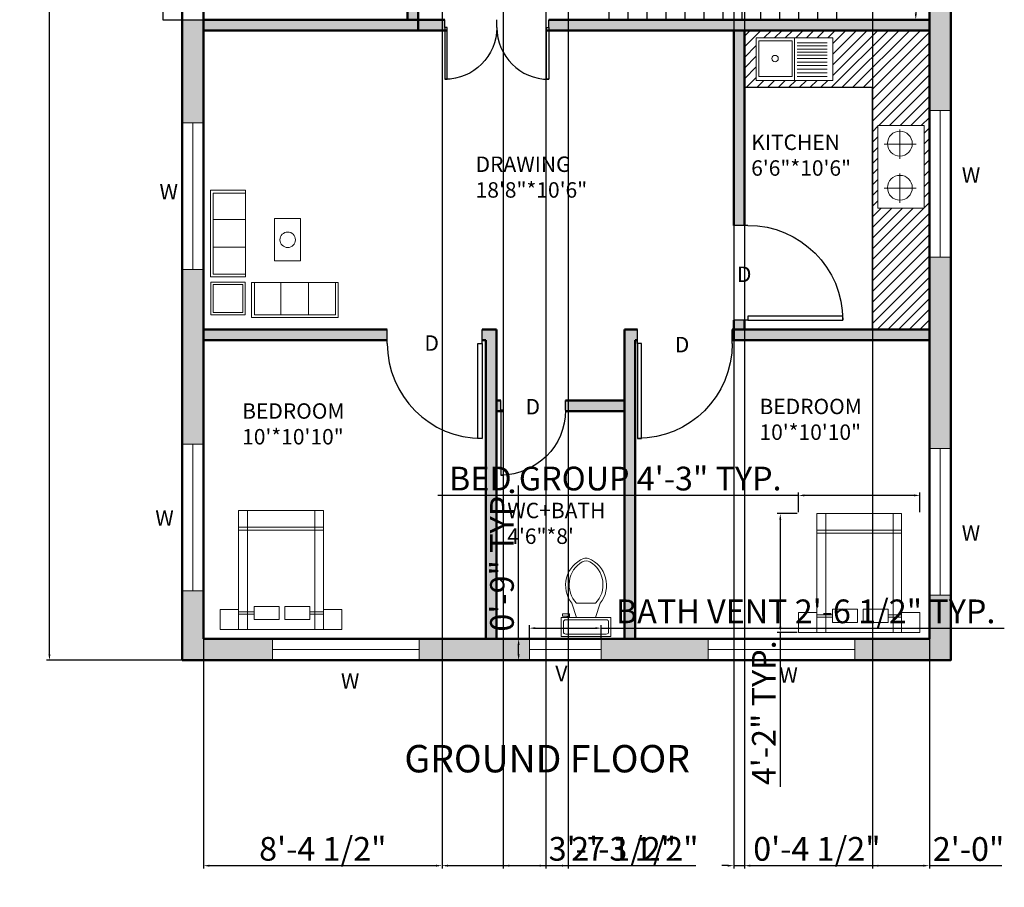
# Model space of a CAD drawing. Units: inches. Extents: x 1935 to 2445, y 1978 to 2806.
# Tile 1 of 4: x 1942 to 2357, y 1978 to 2344. Entities that reach past the tile are written whole.
import ezdxf

# ---------------------------------------------------------------- set-up
doc = ezdxf.new("R2010")
doc.units = ezdxf.units.IN
for name, color, linetype, lineweight in [('A-ANNO-DIMS', 2, 'Continuous', 18), ('A-ANNO-TEXT', 7, 'Continuous', 25), ('A-AREA-IDEN', 130, 'Continuous', 25), ('A-DOOR', 3, 'Continuous', 25), ('A-EQPM', 8, 'Continuous', 18), ('A-FLOR-CASE', 123, 'Continuous', 25), ('A-FLOR-CASE-PATT', 123, 'Continuous', 13), ('A-FLOR-FIXT', 9, 'Continuous', 18), ('A-FLOR-OTLN', 7, 'Continuous', 25), ('A-FLOR-STRS', 7, 'Continuous', 25), ('A-FURN', 9, 'Continuous', 18), ('A-GLAZ', 4, 'Continuous', 18), ('A-WALL-PATT', 225, 'Continuous', 13), ('SOFA', 10, 'Continuous', 18), ('WALL', 225, 'Continuous', 50)]:
    doc.layers.add(name, color=color, linetype=linetype, lineweight=lineweight)
doc.styles.get("Standard").update_dxf_attribs({"font": 'arial.ttf'})
doc.dimstyles.new('ISO-25', dxfattribs={"dimtxt": 10, "dimasz": 2.5, "dimexe": 1.25, "dimexo": 0.625, "dimtad": 1, "dimdec": 0, "dimlunit": 4, "dimtxsty": 'Standard', "dimcen": 2.5, "dimadec": 0, "dimazin": 0, "dimtfac": 1, "dimtdec": 0, "dimtmove": 0, "dimatfit": 3, "dimfxl": 1, "dimarcsym": 0})

# ---------------------------------------------------------------- blocks, each defined once
blk = doc.blocks.new('*U2')
for p, q in [((0, 0), (0, -6)), ((40, 0), (40, -6))]:
    blk.add_line(p, q)
blk.add_lwpolyline([(0, 0), (0, 40), (1.75, 40), (1.75, 0)], close=True)
blk.add_arc((0, 0), 40, 0, 90)
blk = doc.blocks.new('*U4')
for p, q in [((9.5, -6), (9.5, -2)), ((-8, -8.5), (-8, -8)), ((-7, -8), (-7, -9.5)), ((-4, -8), (-6, -14)), ((4, -8), (6, -14)), ((-10, -8.5), (-8, -8.5)), ((-10, -9.5), (-10, -8.5)), ((-7, -9.5), (-10, -9.5)), ((4, -14), (-4, -14))]:
    blk.add_line(p, q)
blk.add_lwpolyline([(10.5, -8), (10.5, 0), (-10.5, 0), (-10.5, -8)], close=True)
for points in [[(-9.5, -2), (-9.5, -6)], [(8.5, -1), (-8.5, -1)], [(-8.5, -7), (8.5, -7)]]:
    blk.add_lwpolyline(points)
for centre, radius, start, end in [((-8.62, -1.88), 0.884, 81.8699, 188.1301), ((8.62, -1.88), 0.884, 351.8699, 98.1301), ((-8.62, -6.12), 0.884, 171.8699, 278.1301), ((8.62, -6.12), 0.884, 261.8699, 8.1301), ((3.52, -21.58), 12.17, 141.4691, 247.9714), ((4.2, -21.82), 11.33, 136.3677, 238.9468), ((-3.52, -21.58), 12.17, 292.0284, 38.5307), ((-4.2, -21.82), 11.33, 301.053, 43.6321), ((0, -27.88), 4, 245.7318, 294.2682), ((0, -29), 4, 254.8605, 285.1395)]:
    blk.add_arc(centre, radius, start, end)
blk = doc.blocks.new('*D7')
at = {"layer": 'A-ANNO-DIMS', "color": 0, "lineweight": -2, "transparency": 16777216}
for p, q in [((2324.56, 2423.88), (2318.18, 2423.88)), ((2319.43, 2421.38), (2319.43, 2346.38)), ((2324.56, 2343.88), (2318.18, 2343.88))]:
    blk.add_line(p, q, dxfattribs=at)
at = {"layer": 'A-ANNO-DIMS', "color": 0, "lineweight": 100, "transparency": 16777216}
for points in [[(2319.01, 2421.38), (2319.85, 2421.38), (2319.43, 2423.88)], [(2319.01, 2346.38), (2319.85, 2346.38), (2319.43, 2343.88)]]:
    blk.add_solid(points, dxfattribs=at)
at = {"layer": 'Defpoints', "color": 0, "lineweight": 100, "transparency": 16777216}
for p in [(2325.18, 2423.88), (2319.43, 2343.88), (2325.18, 2343.88)]:
    blk.add_point(p, dxfattribs=at)
at = {"layer": 'A-ANNO-DIMS', "color": 0, "transparency": 16777216, "insert": (2313.7, 2383.88), "char_height": 10, "attachment_point": 5, "rotation": 90}
blk.add_mtext('6\'-8"', dxfattribs=at)
blk = doc.blocks.new('*D9')
at = {"layer": 'A-ANNO-DIMS', "color": 0, "lineweight": -2, "transparency": 16777216}
for p, q in [((2333.56, 2697.88), (1952.98, 2697.88)), ((1954.23, 2076.38), (1954.23, 2695.38)), ((2333.56, 2073.88), (1952.98, 2073.88))]:
    blk.add_line(p, q, dxfattribs=at)
at = {"layer": 'A-ANNO-DIMS', "color": 0, "lineweight": 100, "transparency": 16777216}
for points in [[(1953.82, 2695.38), (1954.65, 2695.38), (1954.23, 2697.88)], [(1953.82, 2076.38), (1954.65, 2076.38), (1954.23, 2073.88)]]:
    blk.add_solid(points, dxfattribs=at)
at = {"layer": 'Defpoints', "color": 0, "lineweight": 100, "transparency": 16777216}
for p in [(1954.23, 2697.88), (2334.18, 2697.88), (2334.18, 2073.88)]:
    blk.add_point(p, dxfattribs=at)
at = {"layer": 'A-ANNO-DIMS', "color": 0, "transparency": 16777216, "insert": (1948.5, 2385.88), "char_height": 10, "attachment_point": 5, "rotation": 90}
blk.add_mtext("52'", dxfattribs=at)
blk = doc.blocks.new('WINDOW-STD')
blk.add_line((0, 4.5), (61.82, 4.5))
blk.add_lwpolyline([(0, 9), (61.82, 9), (61.82, 0), (0, 0)], close=True)
blk = doc.blocks.new('VENT-BATH')
blk.add_line((0, 4.5), (30.29, 4.5))
blk.add_lwpolyline([(0, 0), (30.29, 0), (30.29, 9), (0, 9)], close=True)
blk = doc.blocks.new('BED-WITH-NIGHTSTANDS')
for p, q in [((11.32, 50.11), (11.32, 0)), ((39.64, 0), (39.64, 50.11)), ((13.46, 43.65), (7.73, 43.65)), ((13.46, 42.6), (7.73, 42.6)), ((43.47, 43.65), (36.85, 43.65)), ((43.47, 42.6), (36.85, 42.6)), ((7.73, 8.18), (43.47, 8.18)), ((7.73, 6.93), (43.47, 6.93)), ((43.47, 0), (39.64, 0))]:
    blk.add_line(p, q)
for points in [[(0, 50.11), (7.73, 50.11), (7.73, 41.64), (0, 41.64)], [(7.73, 50.11), (43.47, 50.11), (43.47, 0), (7.73, 0)], [(43.47, 50.11), (51.2, 50.11), (51.2, 41.64), (43.47, 41.64)], [(13.46, 45.91), (23.93, 45.91), (23.93, 40.33), (13.46, 40.33)], [(26.4, 45.91), (36.86, 45.91), (36.86, 40.33), (26.4, 40.33)]]:
    blk.add_lwpolyline(points, close=True)
blk = doc.blocks.new('SOFA-3-SEAT')
for p, q in [((0, 0), (0, 14.72)), ((0, 14.72), (36.65, 14.72)), ((12.37, 13.53), (12.37, 0)), ((24.09, 13.53), (24.09, 0)), ((36.65, 14.72), (36.65, 0)), ((1.26, 0), (0, 0)), ((36.65, 0), (31.67, 0))]:
    blk.add_line(p, q)
blk.add_lwpolyline([(1.26, 0), (35.43, 0), (35.43, 13.53), (1.26, 13.53)], close=True)
blk = doc.blocks.new('TABLE-END')
for points in [[(0, 13.76), (14.51, 13.76), (14.51, 0), (0, 0)], [(1, 12.76), (13.51, 12.76), (13.51, 1), (1, 1)]]:
    blk.add_lwpolyline(points, close=True)
blk = doc.blocks.new('TABLE-COFFEE')
blk.add_lwpolyline([(0, 0), (10.92, 0), (10.92, 17.81), (0, 17.81)], close=True)
blk.add_circle((5.5, 9), 3.27)
blk = doc.blocks.new('SINK-WITH-DRAINBOARD')
for p, q in [((16.15, 17.9), (16.15, 0)), ((17.28, 15.79), (29.84, 15.79)), ((17.28, 14.55), (29.84, 14.55)), ((17.28, 13.18), (29.84, 13.18)), ((17.28, 11.91), (29.84, 11.91)), ((17.28, 10.66), (29.84, 10.66)), ((17.28, 9.26), (29.84, 9.26)), ((17.28, 7.74), (29.84, 7.74)), ((17.28, 6.29), (29.84, 6.29)), ((17.28, 4.78), (29.84, 4.78)), ((17.28, 3.21), (29.84, 3.21)), ((17.28, 1.68), (29.84, 1.68))]:
    blk.add_line(p, q)
for points in [[(0, 17.9), (32.3, 17.9), (32.3, 0), (0, 0)], [(1.08, 1.69), (15.15, 1.69), (15.15, 16.69), (1.08, 16.69)]]:
    blk.add_lwpolyline(points, close=True)
blk.add_circle((7.93, 9.19), 1.34)
blk = doc.blocks.new('COOKTOP-2-BURNER')
for p, q in [((9.23, 27.22), (9.23, 33.16)), ((9.23, 33.16), (9.23, 20.87)), ((9.23, 27.02), (2.64, 27.02)), ((2.64, 27.02), (16.07, 27.02)), ((9.23, 20.87), (9.23, 27.02)), ((9.23, 8.61), (9.23, 14.56)), ((9.23, 14.56), (9.23, 2.26)), ((9.23, 8.41), (2.64, 8.41)), ((2.64, 8.41), (16.07, 8.41)), ((9.23, 2.26), (9.23, 8.41))]:
    blk.add_line(p, q)
blk.add_lwpolyline([(0, 34.88), (19.51, 34.88), (19.51, 0), (0, 0)], close=True)
for centre in [(9.23, 27.22), (9.23, 8.61)]:
    blk.add_circle(centre, 5.23)
blk = doc.blocks.new('*D20')
at = {"layer": 'A-ANNO-DIMS', "color": 0, "lineweight": -2, "transparency": 16777216}
for p, q in [((2270, 2143.39), (2118.02, 2143.39)), ((2270, 2136.33), (2270, 2144.64)), ((2318.7, 2143.39), (2272.5, 2143.39)), ((2321.2, 2136.33), (2321.2, 2144.64))]:
    blk.add_line(p, q, dxfattribs=at)
at = {"layer": 'A-ANNO-DIMS', "color": 0, "lineweight": 100, "transparency": 16777216}
for points in [[(2272.5, 2143.81), (2272.5, 2142.97), (2270, 2143.39)], [(2318.7, 2143.81), (2318.7, 2142.97), (2321.2, 2143.39)]]:
    blk.add_solid(points, dxfattribs=at)
at = {"layer": 'Defpoints', "color": 0, "lineweight": 100, "transparency": 16777216}
for p in [(2270, 2143.39), (2270, 2135.71), (2321.2, 2135.71)]:
    blk.add_point(p, dxfattribs=at)
at = {"layer": 'A-ANNO-DIMS', "color": 0, "transparency": 16777216, "insert": (2192.76, 2149.19), "char_height": 10, "attachment_point": 5}
blk.add_mtext('BED GROUP 4\'-3" TYP.', dxfattribs=at)
blk = doc.blocks.new('*D21')
at = {"layer": 'A-ANNO-DIMS', "color": 0, "lineweight": -2, "transparency": 16777216}
for p, q in [((2269.37, 2135.71), (2261.07, 2135.71)), ((2262.32, 2133.21), (2262.32, 2088.1)), ((2269.37, 2085.6), (2261.07, 2085.6)), ((2262.32, 2085.6), (2262.32, 2020.49))]:
    blk.add_line(p, q, dxfattribs=at)
at = {"layer": 'A-ANNO-DIMS', "color": 0, "lineweight": 100, "transparency": 16777216}
for points in [[(2261.9, 2133.21), (2262.73, 2133.21), (2262.32, 2135.71)], [(2261.9, 2088.1), (2262.73, 2088.1), (2262.32, 2085.6)]]:
    blk.add_solid(points, dxfattribs=at)
at = {"layer": 'Defpoints', "color": 0, "lineweight": 100, "transparency": 16777216}
for p in [(2270, 2135.71), (2262.32, 2085.6), (2270, 2085.6)]:
    blk.add_point(p, dxfattribs=at)
at = {"layer": 'A-ANNO-DIMS', "color": 0, "transparency": 16777216, "insert": (2256.67, 2051.79), "char_height": 10, "attachment_point": 5, "rotation": 90}
blk.add_mtext('4\'-2" TYP.', dxfattribs=at)
blk = doc.blocks.new('*D22')
at = {"layer": 'A-ANNO-DIMS', "color": 0, "lineweight": -2, "transparency": 16777216}
for p, q in [((2156.55, 2083.51), (2156.55, 2088.68)), ((2186.84, 2083.51), (2186.84, 2088.68)), ((2159.05, 2087.43), (2184.34, 2087.43)), ((2186.84, 2087.43), (2356.68, 2087.43))]:
    blk.add_line(p, q, dxfattribs=at)
at = {"layer": 'A-ANNO-DIMS', "color": 0, "lineweight": 100, "transparency": 16777216}
for points in [[(2159.05, 2087.84), (2159.05, 2087.01), (2156.55, 2087.43)], [(2184.34, 2087.84), (2184.34, 2087.01), (2186.84, 2087.43)]]:
    blk.add_solid(points, dxfattribs=at)
at = {"layer": 'Defpoints', "color": 0, "lineweight": 100, "transparency": 16777216}
for p in [(2186.84, 2087.43), (2156.55, 2082.88), (2186.84, 2082.88)]:
    blk.add_point(p, dxfattribs=at)
at = {"layer": 'A-ANNO-DIMS', "color": 0, "transparency": 16777216, "insert": (2273.01, 2093.22), "char_height": 10, "attachment_point": 5}
blk.add_mtext('BATH VENT 2\'-6 1/2" TYP.', dxfattribs=at)
blk = doc.blocks.new('*D23')
at = {"layer": 'A-ANNO-DIMS', "color": 0, "lineweight": -2, "transparency": 16777216}
for p, q in [((2152.01, 2082.88), (2152.01, 2147.59)), ((2155.93, 2082.88), (2150.76, 2082.88)), ((2152.01, 2076.38), (2152.01, 2080.38)), ((2155.93, 2073.88), (2150.76, 2073.88))]:
    blk.add_line(p, q, dxfattribs=at)
at = {"layer": 'A-ANNO-DIMS', "color": 0, "lineweight": 100, "transparency": 16777216}
for points in [[(2151.59, 2080.38), (2152.42, 2080.38), (2152.01, 2082.88)], [(2151.59, 2076.38), (2152.42, 2076.38), (2152.01, 2073.88)]]:
    blk.add_solid(points, dxfattribs=at)
at = {"layer": 'Defpoints', "color": 0, "lineweight": 100, "transparency": 16777216}
for p in [(2152.01, 2082.88), (2156.55, 2082.88), (2156.55, 2073.88)]:
    blk.add_point(p, dxfattribs=at)
at = {"layer": 'A-ANNO-DIMS', "color": 0, "transparency": 16777216, "insert": (2146.28, 2116.49), "char_height": 10, "attachment_point": 5, "rotation": 90}
blk.add_mtext('0\'-9" TYP.', dxfattribs=at)
blk = doc.blocks.new('*D39')
at = {"layer": 'A-ANNO-DIMS', "color": 0, "lineweight": -2, "transparency": 16777216}
for p, q in [((2019.18, 2423.26), (2019.18, 1986.08)), ((2119.73, 2423.26), (2119.73, 1986.08)), ((2021.68, 1987.33), (2117.23, 1987.33))]:
    blk.add_line(p, q, dxfattribs=at)
at = {"layer": 'A-ANNO-DIMS', "color": 0, "lineweight": 100, "transparency": 16777216}
for points in [[(2021.68, 1987.74), (2021.68, 1986.91), (2019.18, 1987.33)], [(2117.23, 1987.74), (2117.23, 1986.91), (2119.73, 1987.33)]]:
    blk.add_solid(points, dxfattribs=at)
at = {"layer": 'Defpoints', "color": 0, "lineweight": 100, "transparency": 16777216}
for p in [(2019.18, 2423.88), (2119.73, 2423.88), (2119.73, 1987.33)]:
    blk.add_point(p, dxfattribs=at)
at = {"layer": 'A-ANNO-DIMS', "color": 0, "transparency": 16777216, "insert": (2069.46, 1993.12), "char_height": 10, "attachment_point": 5}
blk.add_mtext('8\'-4 1/2"', dxfattribs=at)
blk = doc.blocks.new('*D40')
at = {"layer": 'A-ANNO-DIMS', "color": 0, "lineweight": -2, "transparency": 16777216}
for p, q in [((2119.73, 2423.26), (2119.73, 1986.08)), ((2163.45, 2423.26), (2163.45, 1986.08)), ((2122.23, 1987.33), (2160.95, 1987.33)), ((2163.45, 1987.33), (2217.08, 1987.33))]:
    blk.add_line(p, q, dxfattribs=at)
at = {"layer": 'A-ANNO-DIMS', "color": 0, "lineweight": 100, "transparency": 16777216}
for points in [[(2122.23, 1987.74), (2122.23, 1986.91), (2119.73, 1987.33)], [(2160.95, 1987.74), (2160.95, 1986.91), (2163.45, 1987.33)]]:
    blk.add_solid(points, dxfattribs=at)
at = {"layer": 'Defpoints', "color": 0, "lineweight": 100, "transparency": 16777216}
for p in [(2119.73, 2423.88), (2163.45, 2423.88), (2163.45, 1987.33)]:
    blk.add_point(p, dxfattribs=at)
at = {"layer": 'A-ANNO-DIMS', "color": 0, "transparency": 16777216, "insert": (2191.52, 1993.13), "char_height": 10, "attachment_point": 5}
blk.add_mtext('3\'-7 1/2"', dxfattribs=at)
blk = doc.blocks.new('*D42')
at = {"layer": 'A-ANNO-DIMS', "color": 0, "lineweight": -2, "transparency": 16777216}
for p, q in [((2145.55, 2591.86), (2145.55, 1986.08)), ((2172.86, 2592.26), (2172.86, 1986.08)), ((2148.05, 1987.33), (2170.36, 1987.33)), ((2172.86, 1987.33), (2226.66, 1987.33))]:
    blk.add_line(p, q, dxfattribs=at)
at = {"layer": 'A-ANNO-DIMS', "color": 0, "lineweight": 100, "transparency": 16777216}
for points in [[(2148.05, 1987.74), (2148.05, 1986.91), (2145.55, 1987.33)], [(2170.36, 1987.74), (2170.36, 1986.91), (2172.86, 1987.33)]]:
    blk.add_solid(points, dxfattribs=at)
at = {"layer": 'Defpoints', "color": 0, "lineweight": 100, "transparency": 16777216}
for p in [(2145.55, 2592.49), (2172.86, 2592.88), (2172.86, 1987.33)]:
    blk.add_point(p, dxfattribs=at)
at = {"layer": 'A-ANNO-DIMS', "color": 0, "transparency": 16777216, "insert": (2201.01, 1993.13), "char_height": 10, "attachment_point": 5}
blk.add_mtext('2\'-3 1/2"', dxfattribs=at)
blk = doc.blocks.new('*D44')
at = {"layer": 'A-ANNO-DIMS', "color": 0, "lineweight": -2, "transparency": 16777216}
for p, q in [((2325.18, 2454.54), (2325.18, 1986.08)), ((2301.18, 2451.76), (2301.18, 1986.08)), ((2303.68, 1987.33), (2322.68, 1987.33)), ((2325.18, 1987.33), (2355.69, 1987.33))]:
    blk.add_line(p, q, dxfattribs=at)
at = {"layer": 'A-ANNO-DIMS', "color": 0, "lineweight": 100, "transparency": 16777216}
for points in [[(2303.68, 1987.74), (2303.68, 1986.91), (2301.18, 1987.33)], [(2322.68, 1987.74), (2322.68, 1986.91), (2325.18, 1987.33)]]:
    blk.add_solid(points, dxfattribs=at)
at = {"layer": 'Defpoints', "color": 0, "lineweight": 100, "transparency": 16777216}
for p in [(2325.18, 2455.16), (2301.18, 2452.38), (2325.18, 1987.33)]:
    blk.add_point(p, dxfattribs=at)
at = {"layer": 'A-ANNO-DIMS', "color": 0, "transparency": 16777216, "insert": (2341.69, 1993.06), "char_height": 10, "attachment_point": 5}
blk.add_mtext('2\'-0"', dxfattribs=at)
blk = doc.blocks.new('*D45')
at = {"layer": 'A-ANNO-DIMS', "color": 0, "lineweight": -2, "transparency": 16777216}
for p, q in [((2242.68, 2510.08), (2242.68, 1986.08)), ((2247.18, 2510.08), (2247.18, 1986.08)), ((2240.18, 1987.33), (2237.68, 1987.33)), ((2242.68, 1987.33), (2247.18, 1987.33)), ((2249.68, 1987.33), (2303.32, 1987.33))]:
    blk.add_line(p, q, dxfattribs=at)
at = {"layer": 'A-ANNO-DIMS', "color": 0, "lineweight": 100, "transparency": 16777216}
for points in [[(2240.18, 1987.74), (2240.18, 1986.91), (2242.68, 1987.33)], [(2249.68, 1987.74), (2249.68, 1986.91), (2247.18, 1987.33)]]:
    blk.add_solid(points, dxfattribs=at)
at = {"layer": 'Defpoints', "color": 0, "lineweight": 100, "transparency": 16777216}
for p in [(2242.68, 2510.71), (2247.18, 2510.71), (2247.18, 1987.33)]:
    blk.add_point(p, dxfattribs=at)
at = {"layer": 'A-ANNO-DIMS', "color": 0, "transparency": 16777216, "insert": (2277.75, 1993.12), "char_height": 10, "attachment_point": 5}
blk.add_mtext('0\'-4 1/2"', dxfattribs=at)

msp = doc.modelspace()

# ---------------------------------------------------------------- hatches: boundary and pattern name
at = {"layer": 'A-FLOR-CASE-PATT'}
h = msp.add_hatch(dxfattribs=at)
h.set_pattern_fill('ANSI31', color=256)
h.paths.add_polyline_path([(2325.18, 2339.38), (2286.18, 2339.38), (2247.18, 2339.38), (2247.18, 2315.38), (2301.18, 2315.38), (2301.18, 2213.38), (2325.18, 2213.38)])
h.paths.add_polyline_path([(2284.48, 2318.31), (2252.19, 2318.31), (2252.19, 2336.21), (2284.48, 2336.21)], flags=16)
h.paths.add_polyline_path([(2303.5, 2299.32), (2323.01, 2299.32), (2323.01, 2264.44), (2303.5, 2264.44)], flags=16)
h.paths.add_polyline_path([(2317.96, 2291.66, -1), (2307.51, 2291.66, -1)], flags=0)
h.paths.add_polyline_path([(2267.33, 2320), (2253.26, 2320), (2253.26, 2335.01), (2267.33, 2335.01)], flags=0)
h.paths.add_polyline_path([(2258.78, 2327.5, -1), (2261.46, 2327.5, -1)], flags=0)
h.paths.add_polyline_path([(2317.96, 2273.05, -1), (2307.51, 2273.05, -1)], flags=0)
h.paths.add_polyline_path([(2325.18, 2554.38), (2301.18, 2554.38), (2301.18, 2452.38), (2247.18, 2452.38), (2247.18, 2428.38), (2325.18, 2428.38)])
h.paths.add_polyline_path([(2323.01, 2511.98), (2323.01, 2477.1), (2303.5, 2477.1), (2303.5, 2511.98)], flags=16)
h.paths.add_polyline_path([(2317.96, 2504.31, -1), (2307.51, 2504.31, -1)], flags=0)
h.paths.add_polyline_path([(2317.96, 2485.7, -1), (2307.51, 2485.7, -1)], flags=0)
h.paths.add_polyline_path([(2284.48, 2450.03), (2284.48, 2432.13), (2252.19, 2432.13), (2252.19, 2450.03)], flags=16)
h.paths.add_polyline_path([(2267.33, 2448.82), (2267.33, 2433.82), (2253.26, 2433.82), (2253.26, 2448.82)], flags=0)
h.paths.add_polyline_path([(2261.46, 2441.32, -1), (2258.78, 2441.32, -1)], flags=0)
at = {"layer": 'A-WALL-PATT'}
h = msp.add_hatch(color=256, dxfattribs=at)
h.dxf.hatch_style = 1
h.paths.add_polyline_path([(2047.95, 2697.88), (2010.18, 2697.88), (2010.18, 2654.96), (2019.18, 2654.96), (2019.18, 2688.88), (2047.95, 2688.88)], flags=16)
h.paths.add_polyline_path([(2156.17, 2697.88), (2109.77, 2697.88), (2109.77, 2688.88), (2139.18, 2688.88), (2156.17, 2688.88)], flags=17)
h.paths.add_polyline_path([(2231.53, 2697.88), (2186.46, 2697.88), (2186.46, 2688.88), (2231.53, 2688.88)], flags=17)
h.paths.add_polyline_path([(2334.18, 2697.88), (2293.35, 2697.88), (2293.35, 2688.88), (2325.18, 2688.88), (2325.18, 2651.52), (2334.18, 2651.52)], flags=17)
h.paths.add_polyline_path([(2247.18, 2554.38), (2242.68, 2554.38), (2242.68, 2550.71), (2247.18, 2550.71)], flags=17)
h.paths.add_polyline_path([(2145.55, 2592.49), (2145.55, 2592.88), (2143.68, 2592.88), (2143.68, 2588.39), (2145.55, 2588.39)], flags=17)
h.paths.add_polyline_path([(2197.68, 2592.88), (2172.86, 2592.88, -0.003651), (2172.86, 2592.49), (2172.86, 2588.39), (2197.68, 2588.39)], flags=17)
h.paths.add_polyline_path([(2203.16, 2558.88), (2137.4, 2558.88), (2137.4, 2554.38), (2143.68, 2554.38), (2203.16, 2554.38)], flags=17)
h.paths.add_polyline_path([(2097.4, 2558.88), (2019.18, 2558.88), (2019.18, 2554.38), (2097.4, 2554.38)], flags=17)
h.paths.add_polyline_path([(2143.68, 2688.88), (2139.18, 2688.88), (2139.18, 2558.88), (2143.68, 2558.88)], flags=17)
h.paths.add_polyline_path([(2202.18, 2688.88), (2197.68, 2688.88), (2197.68, 2592.88), (2197.68, 2588.39), (2197.68, 2558.88), (2202.18, 2558.88), (2202.18, 2588.38)], flags=17)
h.paths.add_polyline_path([(2241.74, 2229.79), (2251.55, 2229.79), (2251.55, 2243.19), (2241.74, 2243.19)], flags=25)
h.paths.add_polyline_path([(2215.53, 2200.14), (2225.34, 2200.14), (2225.34, 2213.54), (2215.53, 2213.54)], flags=25)
h.paths.add_polyline_path([(2152.61, 2173.98), (2162.42, 2173.98), (2162.42, 2187.38), (2152.61, 2187.38)], flags=25)
h.paths.add_polyline_path([(2109.99, 2200.78), (2119.8, 2200.78), (2119.8, 2214.18), (2109.99, 2214.18)], flags=25)
h.paths.add_polyline_path([(2139.65, 2343.23), (2149.46, 2343.23), (2149.46, 2356.63), (2139.65, 2356.63)], flags=25)
h.paths.add_polyline_path([(2138.05, 2412.22), (2147.87, 2412.22), (2147.87, 2425.62), (2138.05, 2425.62)], flags=25)
h.paths.add_polyline_path([(2242.1, 2526.57), (2251.91, 2526.57), (2251.91, 2539.97), (2242.1, 2539.97)], flags=25)
h.paths.add_polyline_path([(2212.92, 2555.35), (2222.74, 2555.35), (2222.74, 2568.75), (2212.92, 2568.75)], flags=25)
h.paths.add_polyline_path([(2111.94, 2553.1), (2121.75, 2553.1), (2121.75, 2566.5), (2111.94, 2566.5)], flags=25)
h.paths.add_polyline_path([(2032.85, 2161.17), (2083.36, 2161.17), (2083.36, 2185.43), (2032.85, 2185.43)], flags=25)
h.paths.add_polyline_path([(2145.49, 2119.25), (2193.41, 2119.25), (2193.41, 2143.52), (2145.49, 2143.52)], flags=25)
h.paths.add_polyline_path([(2250.93, 2163.1), (2301.44, 2163.1), (2301.44, 2187.36), (2250.93, 2187.36)], flags=25)
h.paths.add_polyline_path([(2247.75, 2274.43), (2290.88, 2274.43), (2290.88, 2298.69), (2247.75, 2298.69)], flags=25)
h.paths.add_polyline_path([(2131.26, 2265.2), (2178.71, 2265.2), (2178.71, 2289.46), (2131.26, 2289.46)], flags=25)
h.paths.add_polyline_path([(2092.71, 2400.61), (2092.71, 2376.16), (2106.11, 2376.16), (2106.11, 2400.61)], flags=25)
h.paths.add_polyline_path([(2173.61, 2396.23), (2189.48, 2396.23), (2189.48, 2409.63), (2173.61, 2409.63)], flags=25)
h.paths.add_polyline_path([(2028.85, 2376.01), (2076.42, 2376.01), (2076.42, 2400.28), (2028.85, 2400.28)], flags=25)
h.paths.add_polyline_path([(2135.3, 2481.1), (2182.75, 2481.1), (2182.75, 2505.37), (2135.3, 2505.37)], flags=25)
h.paths.add_polyline_path([(2249.01, 2476.21), (2292.13, 2476.21), (2292.13, 2500.47), (2249.01, 2500.47)], flags=25)
h.paths.add_polyline_path([(2251.9, 2596.84), (2302.42, 2596.84), (2302.42, 2621.11), (2251.9, 2621.11)], flags=25)
h.paths.add_polyline_path([(2030.66, 2589.83), (2081.18, 2589.83), (2081.18, 2614.09), (2030.66, 2614.09)], flags=25)
h.paths.add_polyline_path([(2019.18, 2593.14), (2010.18, 2593.14), (2010.18, 2520.31), (2019.18, 2520.31)])
h.paths.add_polyline_path([(2010.18, 2164.99), (2019.18, 2164.99), (2019.18, 2238.56), (2010.18, 2238.56)])
h.paths.add_polyline_path([(2048.33, 2073.88), (2048.33, 2082.88), (2019.18, 2082.88), (2019.18, 2103.18), (2010.18, 2103.18), (2010.18, 2073.88)])
h.paths.add_polyline_path([(2156.55, 2073.88), (2156.55, 2082.88), (2110.15, 2082.88), (2110.15, 2073.88)])
h.paths.add_polyline_path([(2231.91, 2073.88), (2231.91, 2082.88), (2186.84, 2082.88), (2186.84, 2073.88)])
h.paths.add_polyline_path([(2047.95, 2688.88), (2047.95, 2697.88), (2010.18, 2697.88), (2010.18, 2654.96), (2019.18, 2654.96), (2019.18, 2688.88)])
h.paths.add_polyline_path([(2109.77, 2697.88), (2109.77, 2688.88), (2156.17, 2688.88), (2156.17, 2697.88)])
h = msp.add_hatch(color=256, dxfattribs=at)
h.dxf.hatch_style = 1
h.paths.add_polyline_path([(2196.68, 2183.38), (2171.78, 2183.38), (2171.78, 2179.29, -0.003687), (2171.78, 2178.88), (2196.68, 2178.88)], flags=17)
h.paths.add_polyline_path([(2144.47, 2183.38), (2142.68, 2183.38), (2142.68, 2178.88), (2144.47, 2178.88), (2144.47, 2179.29)], flags=17)
h.paths.add_polyline_path([(2096.62, 2213.38), (2019.18, 2213.38), (2019.18, 2208.88), (2096.62, 2208.88)], flags=17)
h.paths.add_polyline_path([(2142.68, 2208.88), (2142.68, 2213.38), (2136.62, 2213.38), (2136.62, 2208.88), (2138.18, 2208.88), (2138.18, 2183.38), (2138.18, 2082.88), (2142.68, 2082.88), (2142.68, 2178.88), (2142.68, 2183.38)], flags=17)
h.paths.add_polyline_path([(2201.18, 2208.88), (2202.06, 2208.88), (2202.06, 2213.38), (2196.68, 2213.38), (2196.68, 2204.97), (2196.68, 2082.88), (2201.18, 2082.88)], flags=17)
h.paths.add_polyline_path([(2247.18, 2217.21), (2242.68, 2217.21), (2242.68, 2213.38), (2247.18, 2213.38)], flags=17)
h.paths.add_polyline_path([(2325.18, 2213.38), (2242.68, 2213.38), (2242.68, 2208.88), (2325.18, 2208.88)], flags=17)
h.paths.add_polyline_path([(2247.18, 2339.38), (2242.68, 2339.38), (2242.68, 2257.21), (2247.18, 2257.21)], flags=17)
h.paths.add_polyline_path([(2325.18, 2343.88), (2286.18, 2343.88), (2186.18, 2343.88), (2164.69, 2343.88), (2164.69, 2340.61), (2164.69, 2339.38), (2213.9, 2339.38), (2286.18, 2339.38), (2325.18, 2339.38)], flags=17)
h.paths.add_polyline_path([(2109.68, 2343.88), (2105.18, 2343.88), (2019.18, 2343.88), (2019.18, 2339.38), (2109.68, 2339.38)], flags=17)
h.paths.add_polyline_path([(2120.97, 2340.61), (2120.97, 2343.88), (2109.68, 2343.88), (2109.68, 2339.38), (2120.97, 2339.38)], flags=17)
h.paths.add_polyline_path([(2109.68, 2356.84), (2105.18, 2356.84), (2105.18, 2343.88), (2109.68, 2343.88)], flags=17)
h.paths.add_polyline_path([(2230.51, 2409.48), (2245.95, 2409.48), (2245.95, 2430.09), (2230.51, 2430.09)], flags=25)
h.paths.add_polyline_path([(2289.31, 2409.69), (2322.13, 2409.69), (2322.13, 2430.3), (2289.31, 2430.3)], flags=25)
h.paths.add_polyline_path([(2241.74, 2229.79), (2251.55, 2229.79), (2251.55, 2243.19), (2241.74, 2243.19)], flags=25)
h.paths.add_polyline_path([(2215.53, 2200.14), (2225.34, 2200.14), (2225.34, 2213.54), (2215.53, 2213.54)], flags=25)
h.paths.add_polyline_path([(2152.61, 2173.98), (2162.42, 2173.98), (2162.42, 2187.38), (2152.61, 2187.38)], flags=25)
h.paths.add_polyline_path([(2109.99, 2200.78), (2119.8, 2200.78), (2119.8, 2214.18), (2109.99, 2214.18)], flags=25)
h.paths.add_polyline_path([(2139.65, 2343.23), (2149.46, 2343.23), (2149.46, 2356.63), (2139.65, 2356.63)], flags=25)
h.paths.add_polyline_path([(2138.05, 2412.22), (2147.87, 2412.22), (2147.87, 2425.62), (2138.05, 2425.62)], flags=25)
h.paths.add_polyline_path([(2242.1, 2526.57), (2251.91, 2526.57), (2251.91, 2539.97), (2242.1, 2539.97)], flags=25)
h.paths.add_polyline_path([(2212.92, 2555.35), (2222.74, 2555.35), (2222.74, 2568.75), (2212.92, 2568.75)], flags=25)
h.paths.add_polyline_path([(2151.96, 2587.49), (2161.77, 2587.49), (2161.77, 2600.89), (2151.96, 2600.89)], flags=25)
h.paths.add_polyline_path([(2111.94, 2553.1), (2121.75, 2553.1), (2121.75, 2566.5), (2111.94, 2566.5)], flags=25)
h.paths.add_polyline_path([(2032.85, 2161.17), (2083.36, 2161.17), (2083.36, 2185.43), (2032.85, 2185.43)], flags=25)
h.paths.add_polyline_path([(2145.49, 2119.25), (2193.41, 2119.25), (2193.41, 2143.52), (2145.49, 2143.52)], flags=25)
h.paths.add_polyline_path([(2250.93, 2163.1), (2301.44, 2163.1), (2301.44, 2187.36), (2250.93, 2187.36)], flags=25)
h.paths.add_polyline_path([(2247.75, 2274.43), (2290.88, 2274.43), (2290.88, 2298.69), (2247.75, 2298.69)], flags=25)
h.paths.add_polyline_path([(2131.26, 2265.2), (2178.71, 2265.2), (2178.71, 2289.46), (2131.26, 2289.46)], flags=25)
h.paths.add_polyline_path([(2173.61, 2396.23), (2189.48, 2396.23), (2189.48, 2409.63), (2173.61, 2409.63)], flags=25)
h.paths.add_polyline_path([(2135.3, 2481.1), (2182.75, 2481.1), (2182.75, 2505.37), (2135.3, 2505.37)], flags=25)
h.paths.add_polyline_path([(2249.01, 2476.21), (2292.13, 2476.21), (2292.13, 2500.47), (2249.01, 2500.47)], flags=25)
h.paths.add_polyline_path([(2251.9, 2596.84), (2302.42, 2596.84), (2302.42, 2621.11), (2251.9, 2621.11)], flags=25)
h.paths.add_polyline_path([(2148.05, 2628.52), (2195.98, 2628.52), (2195.98, 2652.78), (2148.05, 2652.78)], flags=25)
h.paths.add_polyline_path([(2030.66, 2589.83), (2081.18, 2589.83), (2081.18, 2614.09), (2030.66, 2614.09)], flags=25)
h.paths.add_polyline_path([(2325.18, 2414.18), (2334.18, 2414.18), (2334.18, 2455.16), (2325.18, 2455.16)])
h.paths.add_polyline_path([(2325.18, 2305.65), (2334.18, 2305.65), (2334.18, 2352.36), (2325.18, 2352.36)])
h.paths.add_polyline_path([(2325.18, 2163.2), (2334.18, 2163.2), (2334.18, 2243.83), (2325.18, 2243.83)])
h.paths.add_polyline_path([(2293.73, 2082.88), (2293.73, 2073.88), (2334.18, 2073.88), (2334.18, 2101.39), (2325.18, 2101.39), (2325.18, 2082.88)])
h.paths.add_polyline_path([(2334.18, 2589.71), (2325.18, 2589.71), (2325.18, 2516.98), (2334.18, 2516.98)])
h.paths.add_polyline_path([(2293.35, 2697.88), (2293.35, 2688.88), (2325.18, 2688.88), (2325.18, 2651.52), (2334.18, 2651.52), (2334.18, 2697.88)])
h.paths.add_polyline_path([(2109.77, 2697.88), (2109.77, 2688.88), (2231.53, 2688.88), (2231.53, 2697.88)])
h.paths.add_polyline_path([(2010.18, 2654.96), (2019.18, 2654.96), (2019.18, 2688.88), (2047.95, 2688.88), (2047.95, 2697.88), (2010.18, 2697.88)])
h.paths.add_polyline_path([(2010.18, 2520.31), (2019.18, 2520.31), (2019.18, 2593.14), (2010.18, 2593.14)])
h = msp.add_hatch(color=256, dxfattribs=at)
h.dxf.hatch_style = 1
h.paths.add_polyline_path([(2334.18, 2589.71), (2325.18, 2589.71), (2325.18, 2516.98), (2334.18, 2516.98)])
h.paths.add_polyline_path([(2325.18, 2558.88), (2240.84, 2558.88), (2240.84, 2554.38), (2325.18, 2554.38)])
h.paths.add_polyline_path([(2119.73, 2427.16), (2119.73, 2428.38), (2019.18, 2428.38), (2019.18, 2423.88), (2119.73, 2423.88)])
h.paths.add_polyline_path([(2230.51, 2409.48), (2245.95, 2409.48), (2245.95, 2430.09), (2230.51, 2430.09)], flags=9)
h.paths.add_polyline_path([(2289.31, 2409.69), (2322.13, 2409.69), (2322.13, 2430.3), (2289.31, 2430.3)], flags=9)
h.paths.add_polyline_path([(2241.74, 2229.79), (2251.55, 2229.79), (2251.55, 2243.19), (2241.74, 2243.19)], flags=9)
h.paths.add_polyline_path([(2215.53, 2200.14), (2225.34, 2200.14), (2225.34, 2213.54), (2215.53, 2213.54)], flags=9)
h.paths.add_polyline_path([(2152.61, 2173.98), (2162.42, 2173.98), (2162.42, 2187.38), (2152.61, 2187.38)], flags=9)
h.paths.add_polyline_path([(2109.99, 2200.78), (2119.8, 2200.78), (2119.8, 2214.18), (2109.99, 2214.18)], flags=9)
h.paths.add_polyline_path([(2139.65, 2343.23), (2149.46, 2343.23), (2149.46, 2356.63), (2139.65, 2356.63)], flags=9)
h.paths.add_polyline_path([(2138.05, 2412.22), (2147.87, 2412.22), (2147.87, 2425.62), (2138.05, 2425.62)], flags=9)
h.paths.add_polyline_path([(2242.1, 2526.57), (2251.91, 2526.57), (2251.91, 2539.97), (2242.1, 2539.97)], flags=9)
h.paths.add_polyline_path([(2212.92, 2555.35), (2222.74, 2555.35), (2222.74, 2568.75), (2212.92, 2568.75)], flags=9)
h.paths.add_polyline_path([(2151.96, 2587.49), (2161.77, 2587.49), (2161.77, 2600.89), (2151.96, 2600.89)], flags=9)
h.paths.add_polyline_path([(2111.94, 2553.1), (2121.75, 2553.1), (2121.75, 2566.5), (2111.94, 2566.5)], flags=9)
h.paths.add_polyline_path([(2032.85, 2161.17), (2083.36, 2161.17), (2083.36, 2185.43), (2032.85, 2185.43)], flags=9)
h.paths.add_polyline_path([(2145.49, 2119.25), (2193.41, 2119.25), (2193.41, 2143.52), (2145.49, 2143.52)], flags=9)
h.paths.add_polyline_path([(2250.93, 2163.1), (2301.44, 2163.1), (2301.44, 2187.36), (2250.93, 2187.36)], flags=9)
h.paths.add_polyline_path([(2247.75, 2274.43), (2290.88, 2274.43), (2290.88, 2298.69), (2247.75, 2298.69)], flags=9)
h.paths.add_polyline_path([(2131.26, 2265.2), (2178.71, 2265.2), (2178.71, 2289.46), (2131.26, 2289.46)], flags=9)
h.paths.add_polyline_path([(2173.61, 2396.23), (2189.48, 2396.23), (2189.48, 2409.63), (2173.61, 2409.63)], flags=9)
h.paths.add_polyline_path([(2135.3, 2481.1), (2182.75, 2481.1), (2182.75, 2505.37), (2135.3, 2505.37)], flags=9)
h.paths.add_polyline_path([(2249.01, 2476.21), (2292.13, 2476.21), (2292.13, 2500.47), (2249.01, 2500.47)], flags=9)
h.paths.add_polyline_path([(2251.9, 2596.84), (2302.42, 2596.84), (2302.42, 2621.11), (2251.9, 2621.11)], flags=9)
h.paths.add_polyline_path([(2148.05, 2628.52), (2195.98, 2628.52), (2195.98, 2652.78), (2148.05, 2652.78)], flags=9)
h.paths.add_polyline_path([(2030.66, 2589.83), (2081.18, 2589.83), (2081.18, 2614.09), (2030.66, 2614.09)], flags=9)
h = msp.add_hatch(color=256, dxfattribs=at)
h.dxf.hatch_style = 1
h.paths.add_polyline_path([(2019.18, 2458.49), (2010.18, 2458.49), (2010.18, 2423.88), (2019.18, 2423.88)])
h.paths.add_polyline_path([(2019.18, 2343.88), (2010.18, 2343.88), (2010.18, 2300.38), (2019.18, 2300.38)])

# ---------------------------------------------------------------- linework, layer by layer
at = {"layer": 'A-FLOR-CASE'}
for p, q in [((2247.18, 2339.38), (2247.18, 2315.38)), ((2247.18, 2315.38), (2301.18, 2315.38)), ((2301.18, 2213.38), (2301.18, 2315.38)), ((2325.18, 2213.38), (2301.18, 2213.38))]:
    msp.add_line(p, q, dxfattribs=at)
at = {"layer": 'A-FLOR-OTLN'}
for p, q in [((2001.98, 2423.88), (2001.98, 2343.88)), ((2001.98, 2343.88), (2028.99, 2343.88))]:
    msp.add_line(p, q, dxfattribs=at)
at = {"layer": 'A-FLOR-STRS'}
for p, q in [((2190.18, 2343.88), (2190.18, 2423.88)), ((2198.18, 2343.88), (2198.18, 2423.88)), ((2206.18, 2343.88), (2206.18, 2423.88)), ((2214.18, 2343.88), (2214.18, 2423.88)), ((2222.18, 2343.88), (2222.18, 2423.88)), ((2230.18, 2343.88), (2230.18, 2423.88)), ((2238.18, 2343.88), (2238.18, 2423.88)), ((2246.18, 2343.88), (2246.18, 2423.88)), ((2254.18, 2343.88), (2254.18, 2423.88)), ((2262.18, 2343.88), (2262.18, 2423.88)), ((2270.18, 2343.88), (2270.18, 2423.88)), ((2278.18, 2343.88), (2278.18, 2423.88)), ((2286.18, 2343.88), (2286.18, 2423.88))]:
    msp.add_line(p, q, dxfattribs=at)
at = {"layer": 'WALL'}
for p, q in [((2325.18, 2423.88), (2325.18, 2343.88)), ((2105.18, 2356.84), (2105.18, 2343.88)), ((2109.68, 2356.84), (2109.68, 2339.38)), ((2105.18, 2343.88), (2019.18, 2343.88)), ((2105.18, 2343.88), (2120.97, 2343.88)), ((2164.69, 2343.88), (2272.65, 2343.88)), ((2286.18, 2343.88), (2186.18, 2343.88)), ((2325.18, 2343.88), (2286.18, 2343.88)), ((2109.68, 2339.38), (2019.18, 2339.38)), ((2109.68, 2339.38), (2121.93, 2339.38)), ((2142.8, 2339.38), (2142.86, 2339.38)), ((2163.73, 2339.38), (2213.9, 2339.38)), ((2286.18, 2339.38), (2186.18, 2339.38)), ((2242.68, 2257.21), (2242.68, 2339.38)), ((2247.18, 2257.21), (2247.18, 2339.38)), ((2325.18, 2339.38), (2286.18, 2339.38)), ((2325.18, 2339.38), (2325.18, 2213.38)), ((2242.68, 2208.88), (2242.68, 2217.21)), ((2247.18, 2213.38), (2247.18, 2217.21)), ((2096.62, 2213.38), (2019.18, 2213.38)), ((2142.68, 2213.38), (2136.62, 2213.38)), ((2142.68, 2208.88), (2142.68, 2213.38)), ((2202.06, 2213.38), (2196.68, 2213.38)), ((2196.68, 2213.38), (2196.68, 2204.97)), ((2325.18, 2213.38), (2242.06, 2213.38)), ((2325.18, 2213.38), (2247.18, 2213.38)), ((2096.62, 2208.88), (2019.18, 2208.88)), ((2138.18, 2208.88), (2136.62, 2208.88)), ((2138.18, 2183.38), (2138.18, 2208.88)), ((2142.68, 2178.88), (2142.68, 2208.88)), ((2196.68, 2208.88), (2196.68, 2082.88)), ((2201.18, 2208.88), (2201.18, 2082.88)), ((2202.06, 2208.88), (2201.18, 2208.88)), ((2325.18, 2208.88), (2242.06, 2208.88)), ((2325.18, 2208.88), (2242.68, 2208.88)), ((2138.18, 2082.88), (2138.18, 2183.38)), ((2142.68, 2183.38), (2144.47, 2183.38)), ((2171.78, 2183.38), (2196.68, 2183.38)), ((2142.68, 2082.88), (2142.68, 2178.88)), ((2142.68, 2178.88), (2145.66, 2178.88)), ((2171.78, 2178.88), (2196.68, 2178.88)), ((2196.68, 2082.88), (2142.68, 2082.88)), ((2144.07, 2073.88), (2198.07, 2073.88))]:
    msp.add_line(p, q, dxfattribs=at)
for points in [[(2010.18, 2073.88), (2334.18, 2073.88), (2334.18, 2697.88), (2010.18, 2697.88)], [(2019.18, 2082.88), (2325.18, 2082.88), (2325.18, 2688.88), (2019.18, 2688.88)]]:
    msp.add_lwpolyline(points, close=True, dxfattribs=at)

# ---------------------------------------------------------------- block references
at = {"layer": 'A-DOOR', "rotation": 180}
for p, xscale, yscale, zscale in [((2120.97, 2340.61), -0.5464986949645749, 0.5464986949645749, 0.5464986949645749), ((2164.69, 2340.61), 0.5464986949645749, 0.5464986949645749, 0.5464986949645749), ((2144.47, 2179.29), -0.6828645758789585, 0.6828645758789585, 0.6828645758789585)]:
    msp.add_blockref('*U2', p, dxfattribs=dict(at, xscale=xscale, yscale=yscale, zscale=zscale))
at = {"layer": 'A-DOOR', "xscale": -1}
for p, rotation in [((2248.68, 2217.21), 270), ((2202.06, 2207.38), 180)]:
    msp.add_blockref('*U2', p, dxfattribs=dict(at, rotation=rotation))
at = {"layer": 'A-DOOR', "rotation": 180}
msp.add_blockref('*U2', (2136.62, 2207.38), dxfattribs=at)
at = {"layer": 'A-EQPM'}
msp.add_blockref('COOKTOP-2-BURNER', (2303.5, 2264.44), dxfattribs=at)
at = {"layer": 'A-FLOR-FIXT'}
msp.add_blockref('SINK-WITH-DRAINBOARD', (2252.19, 2318.31), dxfattribs=at)
at = {"layer": 'A-FLOR-FIXT', "xscale": -1, "rotation": 180}
msp.add_blockref('*U4', (2180.45, 2083.93), dxfattribs=at)
at = {"layer": 'A-FURN', "extrusion": (0, 0, -1), "zscale": -1, "rotation": 180}
for name, p in [('TABLE-COFFEE', (-2049.17, 2260.11)), ('TABLE-END', (-2022.21, 2233.25))]:
    msp.add_blockref(name, p, dxfattribs=at)
at = {"layer": 'A-FURN', "rotation": 180}
for p in [(2077.42, 2136.96), (2321.2, 2135.71)]:
    msp.add_blockref('BED-WITH-NIGHTSTANDS', p, dxfattribs=at)
at = {"layer": 'A-GLAZ'}
for p, rotation in [((2325.18, 2305.65), 270.0000000000007), ((2010.18, 2300.38), 270.0000000000002), ((2010.18, 2165), 270.0000000000002), ((2325.18, 2163.2), 270.0000000000005)]:
    msp.add_blockref('WINDOW-STD', p, dxfattribs=dict(at, rotation=rotation))
for name, p in [('WINDOW-STD', (2048.33, 2073.88)), ('VENT-BATH', (2156.55, 2073.88)), ('WINDOW-STD', (2231.91, 2073.88))]:
    msp.add_blockref(name, p, dxfattribs=at)
at = {"layer": 'SOFA', "extrusion": (0, 0, -1), "zscale": -1}
for p, rotation in [((-2036.82, 2272.09), 270.0000000000017), ((-2039.35, 2233.05), 180)]:
    msp.add_blockref('SOFA-3-SEAT', p, dxfattribs=dict(at, rotation=rotation))

# ---------------------------------------------------------------- texts
at = {"layer": 'A-ANNO-TEXT', "attachment_point": 1}
for s, width, gutter_width, insert, char_height in [('W', 118.8911, 32.51, (2338.84, 2281.67), 6.5), ('W', 118.8911, 32.51, (2000.63, 2274.61), 6.5), ('D', 118.8911, 32.51, (2244.06, 2239.85), 6.5), ('D', 118.8911, 32.51, (2112.31, 2210.83), 6.5), ('D', 118.8911, 32.51, (2217.85, 2210.19), 6.5), ('D', 118.8911, 32.51, (2154.94, 2184.03), 6.5), ('W', 118.8911, 32.51, (1998.85, 2137.11), 6.5), ('W', 118.8911, 32.51, (2338.8, 2130.82), 6.5), ('V', 118.8911, 32.51, (2167.5, 2071.56), 6.5), ('W', 118.8911, 32.51, (2077.1, 2068.46), 6.5), ('W', 118.8911, 32.51, (2261.92, 2070.9), 6.5), ('GROUND FLOOR', 978.8337, 57.79, (2103.86, 2038.2), 11.5582)]:
    msp.add_mtext_dynamic_manual_height_columns(s, width=width, gutter_width=gutter_width, heights=[0], dxfattribs=dict(at, insert=insert, char_height=char_height))
at = {"layer": 'A-AREA-IDEN', "attachment_point": 1}
for s, insert, char_height in [('KITCHEN\\P6\'6"*10\'6"', (2250.05, 2295.46), 6.503), ('DRAWING\\P18\'8"*10\'6"', (2133.88, 2286.22), 6.5027), ('BEDROOM\\P10\'*10\'10"', (2253.54, 2184.13), 6.503), ('BEDROOM\\P10\'*10\'10"', (2035.46, 2182.2), 6.503), ('WC+BATH\\P4\'6"*8\'', (2147.23, 2140.28), 6.503)]:
    msp.add_mtext_dynamic_manual_height_columns(s, width=118.8911, gutter_width=32.51, heights=[0], dxfattribs=dict(at, insert=insert, char_height=char_height))

# ---------------------------------------------------------------- dimensions: what is measured, and where the dimension line sits
at = {"layer": 'A-ANNO-DIMS'}
for base, p1, p2, picture, middle in [((1954.23, 2697.88), (2334.18, 2073.88), (2334.18, 2697.88), '*D9', (1948.5, 2385.88)), ((2319.43, 2343.88), (2325.18, 2423.88), (2325.18, 2343.88), '*D7', (2313.7, 2383.88))]:
    dim = msp.add_linear_dim(base=base, p1=p1, p2=p2, angle=90, dimstyle='ISO-25', override={"dimclrd": 0, "dimclre": 0, "dimclrt": 0}, dxfattribs=at)
    dim.commit()
    dim.dimension.update_dxf_attribs({"geometry": picture, "text_midpoint": middle})
for base, p1, p2, picture, middle in [((2172.86, 1987.33), (2145.55, 2592.49), (2172.86, 2592.88), '*D42', (2201.01, 1993.13)), ((2247.18, 1987.33), (2242.68, 2510.71), (2247.18, 2510.71), '*D45', (2277.75, 1993.12)), ((2325.18, 1987.33), (2301.18, 2452.38), (2325.18, 2455.16), '*D44', (2341.69, 1993.06)), ((2119.7319, 1987.3265), (2019.1844, 2423.8842), (2119.7319, 2423.8842), '*D39', (2069.4582, 1993.1221)), ((2163.45, 1987.33), (2119.73, 2423.88), (2163.45, 2423.88), '*D40', (2191.52, 1993.13))]:
    dim = msp.add_linear_dim(base=base, p1=p1, p2=p2, dimstyle='ISO-25', override={"dimdec": 1, "dimlfac": 1, "dimrnd": 0, "dimzin": 1, "dimdsep": 46, "dimlunit": 4, "dimfrac": 2}, dxfattribs=at)
    dim.commit()
    dim.dimension.update_dxf_attribs({"geometry": picture, "text_midpoint": middle})
for base, p1, p2, angle, text, picture, middle in [((2270, 2143.39), (2321.2, 2135.71), (2270, 2135.71), 180, 'BED GROUP <> TYP.', '*D20', (2192.76, 2149.19)), ((2152.01, 2082.88), (2156.55, 2073.88), (2156.55, 2082.88), 90, '<> TYP.', '*D23', (2146.28, 2116.49)), ((2262.32, 2085.6), (2270, 2135.71), (2270, 2085.6), 270, '<> TYP.', '*D21', (2256.67, 2051.79))]:
    dim = msp.add_linear_dim(base=base, p1=p1, p2=p2, angle=angle, text=text, dimstyle='ISO-25', override={"dimdec": 1, "dimlfac": 1, "dimrnd": 0, "dimzin": 1, "dimdsep": 46, "dimlunit": 4, "dimfrac": 2}, dxfattribs=at)
    dim.commit()
    dim.dimension.update_dxf_attribs({"geometry": picture, "text_midpoint": middle})
dim = msp.add_linear_dim(base=(2186.84, 2087.43), p1=(2156.55, 2082.88), p2=(2186.84, 2082.88), text='BATH VENT <> TYP.', dimstyle='ISO-25', override={"dimdec": 1, "dimlfac": 1, "dimrnd": 0, "dimzin": 1, "dimdsep": 46, "dimlunit": 4, "dimfrac": 2}, dxfattribs=at)
dim.commit()
dim.dimension.update_dxf_attribs({"geometry": '*D22', "text_midpoint": (2273.01, 2093.22)})

doc.saveas('drawing.dxf')
